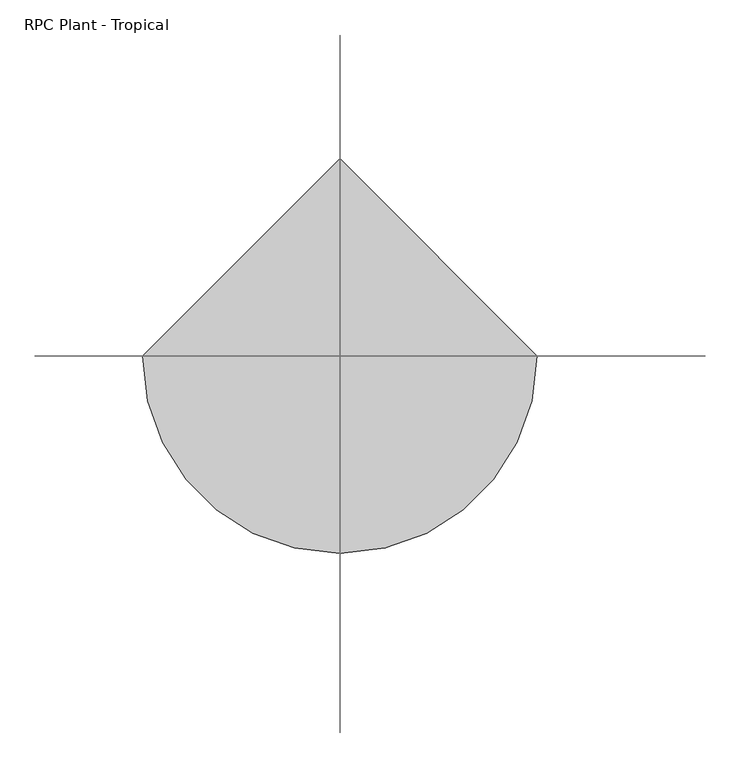
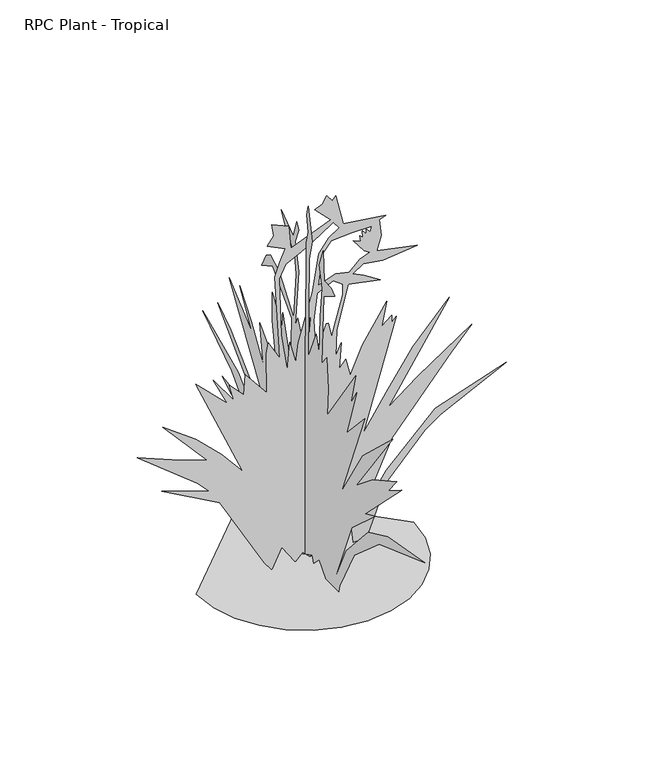
"""IFC4 building model written with IfcOpenShell, lengths in millimetres: geographic element geometry, RPC Plant - Tropical."""

from ifc_helpers import new_model, si_unit, origin, place, context, project, spatial, triangles, source, transform, mapped, element, save


def rpc_plant_tropical_5a024449(model_context):
    return source(origin(), model_context, "Body", "Tessellation", [
        triangles([(-352.4506888, 0.0, 0.0363366), (-343.133961, -80.7585154, 0.0363366), (-316.5967, -154.9221753, 0.0363366), (-274.9660652, -220.3661821, 0.0363366), (-220.3661821, -274.9660652, 0.0363366), (-154.9221753, -316.5967, 0.0363366), (-80.7585154, -343.133961, 0.0363366), (1.54e-05, -352.4506888, 0.0363366), (80.7585154, -343.133961, 0.0363366), (154.9221753, -316.5967, 0.0363366), (220.3661821, -274.9660652, 0.0363366), (274.9660652, -220.3661821, 0.0363366), (316.5967, -154.9221753, 0.0363366), (343.133961, -80.7585154, 0.0363366), (352.4506888, 3.08e-05, 0.0363366), (-4.62e-05, 352.4506888, 0.0363366), (-7e-06, -188.4942358, 0.0), (-3.7e-06, -119.2212567, 0.072664), (-4.19e-05, -79.9125278, 44.364693), (-4.14e-05, -48.5103157, 13.1292711), (-4.04e-05, -40.4507195, 34.8461175), (2.9e-06, 29.5134692, 0.0471628), (-3.66e-05, 46.7858207, 29.9671479), (-3.6e-05, 67.2433383, 18.6432763), (-3.21e-05, 95.7370796, 107.7136924), (7e-06, 122.150729, 0.0282337), (-3.15e-05, 145.3538185, 54.4566279), (-3.22e-05, 150.4477027, 21.3286672), (-2.45e-05, 219.2584009, 179.4152478), (-2e-05, 268.4033662, 254.4167563), (-1.15e-05, 419.8623445, 314.6778128), (-8.6e-06, 464.3123566, 343.8315928), (-1.17e-05, 402.021355, 334.0278671), (-1.57e-05, 328.9766493, 309.2787601), (-9.5e-06, 412.0797526, 393.381984), (1e-06, 573.7356557, 502.2058285), (-1.06e-05, 373.9628205, 412.4692274), (-2.11e-05, 232.7566504, 272.4267398), (-1.31e-05, 320.2214424, 409.8716752), (-4e-07, 490.2271628, 579.950211), (-5.1e-06, 416.7906206, 532.3505728), (-1.51e-05, 280.1801728, 400.4499393), (-2.2e-05, 197.5793099, 294.4509224), (-1.56e-05, 249.5602758, 431.0688189), (5e-07, 426.8795033, 703.7701967), (-8.6e-06, 297.3021655, 594.3503131), (-2e-06, 366.4105199, 712.4096403), (-7.3e-06, 302.3066384, 630.5538082), (-1.36e-05, 233.9534886, 522.3632827), (-8.7e-06, 254.1095984, 654.8193329), (-1.6e-05, 159.0860926, 554.0354047), (-1.04e-05, 183.2709718, 706.1374941), (-7.4e-06, 185.0015529, 801.6720697), (-1.26e-05, 126.6018291, 714.9293266), (-1.12e-05, 124.5318973, 767.1178562), (-1.76e-05, 79.4309438, 617.9316862), (-1.3e-05, 74.9422506, 778.5851068), (-4.9e-06, 181.3398942, 892.1909632), (-3.1e-06, 242.5915333, 859.2623772), (-2.8e-06, 218.5658196, 907.5833376), (-3.4e-06, 196.0532766, 922.0681366), (-6.5e-06, 144.2406234, 895.875622), (-1.33e-05, 64.0625777, 787.2753468), (-9.2e-06, 49.1612298, 945.4327715), (-7e-06, 58.4837167, 1004.946726), (-2.6e-06, 111.6686472, 1072.5920883), (-4e-07, 133.1706141, 1115.5383768), (-4.9e-06, 65.5147783, 1066.5197845), (-3.9e-06, 46.7858207, 1127.0564964), (-5.1e-06, 35.2674194, 1104.0203299), (-5.7e-06, 55.4238608, 1055.069466), (-9.3e-06, 35.7994659, 961.6447906), (-1.43e-05, 55.4238608, 767.1178562), (-1.4e-05, 41.026452, 798.7933937), (-1.71e-05, 12.2314311, 735.4457342), (-1.69e-05, -5.6583455, 769.5562975), (-7.6e-06, -8.3749288, 1087.6424051), (-6.7e-06, -18.0932474, 1129.9351725), (-4.7e-06, -9.2615923, 1183.6781857), (-4.1e-06, -19.4430719, 1219.2010174), (-8.3e-06, -40.4002548, 1110.9765913), (-9.6e-06, -22.855107, 1040.9876947), (-1.95e-05, -19.4430719, 703.7701967), (-1.83e-05, -62.6354346, 807.4327646), (-2.09e-05, -79.9125278, 746.9637812), (-1.71e-05, -85.0409575, 882.7455368), (-1.46e-05, -98.1639664, 984.6876429), (-1.17e-05, -79.9125278, 1055.069466), (-1.13e-05, -91.4305929, 1086.7449308), (-1.09e-05, -102.9486489, 1118.4170528), (-1.41e-05, -108.7076815, 1017.6365765), (-1.59e-05, -147.9066878, 1015.7603828), (-1.73e-05, -168.637163, 1002.06805), (-1.64e-05, -133.7778445, 980.3865973), (-1.57e-05, -106.2777517, 962.7454502), (-2.22e-05, -94.3099411, 726.8063633), (-2.24e-05, -123.1863762, 763.1148302), (-2.58e-05, -131.7434665, 660.5766123), (-2.83e-05, -125.984443, 568.4321277), (-2.85e-05, -284.3569528, 798.7933937), (-3.06e-05, -258.4414743, 689.3734737), (-3.04e-05, -290.1159762, 744.0817623), (-3.3e-05, -235.4056892, 574.1928589), (-3.43e-05, -336.1882367, 683.6127789), (-3.82e-05, -203.7311873, 352.4710001), (-3.78e-05, -325.8775289, 550.7232522), (-4.05e-05, -492.4352766, 708.0950054), (-3.98e-05, -287.2366462, 424.4580305), (-4.17e-05, -380.6345427, 501.4810544), (-4.55e-05, -516.7854255, 575.8116918), (-4.52e-05, -468.6439236, 516.6025515), (-4.71e-05, -542.6155712, 562.8170271), (-4.4e-05, -338.802394, 359.1257901), (-4.58e-05, -393.7782171, 384.1465376), (-4.35e-05, -263.4686565, 265.0881616), (-4.64e-05, -157.658945, 9.8106396), (-4.49e-05, -230.9356314, 167.2679333), (-4.64e-05, -355.769636, 306.2348325), (-4.97e-05, -463.9838519, 356.4029185), (-5.8e-05, -673.0903833, 392.7859085), (-4.92e-05, -416.1708547, 301.7891554), (-4.67e-05, -276.4290936, 178.0792102), (-4.76e-05, -195.0924704, 24.2081495), (156.4407599, 3.08e-05, 0.0540164), (147.1186091, 2.78e-05, 99.2121401), (104.1123133, 3.39e-05, 28.0194403), (74.1534952, 3.32e-05, 61.6417861), (16.7830803, 3.86e-05, 0.0163075), (-6.8943443, 3.9e-05, 24.1987001), (-32.13939, 4.12e-05, 0.0049902), (-75.5809789, 3.96e-05, 64.5211298), (-108.2819807, 4.37e-05, 0.0242217), (-131.9818967, 4.4e-05, 32.1918168), (-277.0556361, 3.5e-05, 288.8520817), (-464.3123566, 3.7e-05, 392.7859085), (-311.6995789, 3.34e-05, 340.9529531), (-348.8032371, 3.27e-05, 380.3771456), (-544.9387942, 3.2e-05, 536.7600057), (-432.90439, 2.98e-05, 490.7182302), (-317.4586023, 2.73e-05, 447.4941607), (-461.4337169, 2.38e-05, 611.6257484), (-354.9737543, 2.38e-05, 533.6239326), (-271.765988, 2.5e-05, 452.9534932), (-202.2786415, 2.69e-05, 369.7497783), (-354.8924729, 1.27e-05, 721.0455957), (-252.5181985, 1.41e-05, 621.3522623), (-297.3021655, 1.05e-05, 715.2882437), (-231.6454718, 1.31e-05, 622.9033304), (-245.4708816, 1.03e-05, 680.7341028), (-199.3989663, 1.12e-05, 631.7831663), (-193.6399246, 7e-06, 698.0128447), (-124.5318973, 9.1e-06, 611.6257484), (-125.4645892, 1.2e-06, 745.9139179), (-118.7732008, -1.3e-06, 781.5179947), (-81.3393302, 1.1e-06, 715.2882437), (-85.8974459, -2.5e-06, 778.2870872), (-97.8195379, -1.51e-05, 999.0640909), (-82.2889543, -1.85e-05, 1044.4149565), (-63.8773237, -2.17e-05, 1084.6486198), (-121.652549, -2.09e-05, 1112.6597734), (-102.0606671, -2.35e-05, 1141.85959), (-107.2551448, -2.56e-05, 1181.7681278), (-53.1866246, -2.66e-05, 1158.7286184), (-46.7858207, -2.23e-05, 1080.984236), (82.791876, -3.1e-05, 1132.8171913), (30.9610326, -3.18e-05, 1184.6468039), (56.5553461, -3.36e-05, 1195.3351049), (71.2741515, -3.57e-05, 1219.2010174), (88.2593112, -3.5e-05, 1195.8464836), (99.6798441, -3.63e-05, 1209.0409544), (124.9047669, -3.11e-05, 1104.1998247), (261.5829613, -3.6e-05, 1085.2209686), (241.1643857, -3.47e-05, 1078.1055599), (247.6434234, -3.16e-05, 1022.4964542), (232.526014, -2.81e-05, 974.442992), (364.9847348, -3.22e-05, 945.6495461), (252.5110768, -2.66e-05, 934.6123564), (189.4235214, -2.44e-05, 944.2101717), (154.7792516, -2.16e-05, 922.6133795), (190.4700055, -2.22e-05, 905.4700945), (244.0440791, -2.24e-05, 870.7804241), (140.4238415, -1.92e-05, 892.113061), (102.7322468, -8.9e-06, 747.339703), (100.0689646, -3.6e-06, 660.5766123), (117.2288819, -6.7e-06, 699.1914064), (111.5866936, -1.2e-06, 611.6257484), (131.7434665, -3.6e-06, 637.5405184), (146.1408799, -7e-07, 577.0715349), (185.2586048, -7.7e-06, 666.3610703), (265.3438509, -1.85e-05, 789.3445518), (249.8031026, -1.31e-05, 709.5309643), (281.4776045, -1.6e-05, 735.4457342), (281.4776045, -1.46e-05, 712.4096403), (295.8750179, -1.61e-05, 726.8063633), (189.3334469, 1.02e-05, 363.9890471), (263.1983969, 1e-07, 478.5499323), (349.8700324, -1.11e-05, 603.7618752), (468.6439236, -2.4e-05, 732.5637154), (269.9592124, 3e-06, 424.4580305), (365.1879564, -5.5e-06, 496.9700289), (540.6343695, -2.01e-05, 614.5043518), (474.2149861, -1.28e-05, 541.0475347), (282.0360734, 9.1e-06, 313.8541712), (175.5771282, 2.77e-05, 79.3862427), (263.306439, 1.6e-05, 211.1110784), (422.7545371, -2e-07, 366.6882282), (652.9328928, -1.49e-05, 444.6154847), (440.209431, 6e-07, 340.3230134), (389.1045925, 5e-06, 303.7012662), (265.6320601, 1.84e-05, 169.4411655), (197.9718186, 2.84e-05, 0.0676572), (152.5051171, -2.99e-05, 1063.2651867), (84.8953359, -2.67e-05, 1059.6481836), (56.4266521, -2.33e-05, 1023.4176189), (42.4789932, -1.67e-05, 922.6133795), (99.5955106, -2.04e-05, 941.7650448), (143.2615316, -2.16e-05, 931.2494076), (177.0767459, -2.5e-05, 963.6090603), (209.4902289, -2.73e-05, 977.3216681), (191.9066365, -2.72e-05, 988.3689589), (156.7607985, -2.84e-05, 1035.0541906), (181.2907874, -2.89e-05, 1024.4065121), (178.2695329, -2.99e-05, 1044.3201221), (187.5906572, -2.98e-05, 1036.1311598), (186.4540987, -3.11e-05, 1057.9480694), (197.9718186, -3.07e-05, 1043.5513464), (198.4063306, -3.17e-05, 1060.2171896), (211.3004019, -3.15e-05, 1047.3139801), (216.3485676, -3.27e-05, 1063.5597908), (48.6623731, -2.71e-05, 1092.001078), (-14.0239612, -2.21e-05, 1054.3684187), (-62.1379314, -1.86e-05, 1031.511747), (-83.7838303, -1.52e-05, 989.2190523), (-76.8587716, -3.8e-06, 793.0800797), (-58.3035451, 3e-06, 666.3373798), (-49.6651689, -2.9e-06, 758.4818281), (-29.5084913, 7e-07, 683.6127789), (-21.1900174, -3.4e-06, 746.4862667), (24.1221968, -1.47e-05, 902.7268753), (44.8185034, -2.32e-05, 1029.605032), (76.8929719, -2.72e-05, 1073.8553106), (111.5866936, -3e-05, 1095.3809589), (91.4305929, -3.07e-05, 1121.2991444), (40.2783372, -1.5e-05, 895.5437382), (29.068629, -9.2e-06, 806.7283745), (34.2422754, -3.3e-06, 704.1156698), (41.1405802, -3.7e-06, 704.9792799), (68.7334726, -9.5e-06, 781.72118), (74.7695323, -9.7e-06, 780.8609854), (86.8413109, -7.2e-06, 730.846669), (92.8773796, -9.1e-06, 757.5775955), (122.1947579, -1.65e-05, 861.0504948), (122.1947579, -1.87e-05, 897.2675428), (91.1525484, -1.87e-05, 920.5475172), (9.23626, -7.6e-06, 793.7946436), (14.4099058, -6.1e-06, 764.4762297), (17.8590253, -8.2e-06, 797.2423256), (20.4458655, -1.06e-05, 836.0467157)], [[15, 16, 1], [14, 15, 1], [14, 1, 2], [13, 14, 2], [13, 2, 3], [13, 3, 4], [12, 13, 4], [11, 12, 4], [11, 4, 5], [11, 5, 6], [11, 6, 7], [11, 7, 8], [11, 8, 9], [11, 9, 10], [46, 47, 48], [119, 120, 121], [35, 36, 37], [106, 107, 108], [39, 40, 41], [39, 41, 42], [101, 102, 103], [111, 112, 113], [105, 106, 108], [44, 45, 46], [113, 114, 115], [54, 55, 56], [103, 104, 105], [99, 100, 101], [109, 110, 111], [89, 90, 91], [118, 119, 121], [31, 32, 33], [46, 48, 49], [44, 46, 49], [79, 80, 81], [78, 79, 81], [66, 67, 68], [27, 28, 29], [52, 53, 54], [88, 89, 91], [87, 88, 91], [49, 50, 51], [58, 59, 60], [99, 101, 103], [25, 26, 27], [83, 84, 85], [109, 111, 113], [108, 109, 113], [96, 97, 98], [68, 69, 70], [68, 70, 71], [38, 39, 42], [38, 42, 43], [65, 66, 68], [65, 68, 71], [65, 71, 72], [64, 65, 72], [64, 72, 73], [63, 64, 73], [118, 121, 122], [117, 118, 122], [117, 122, 123], [116, 117, 123], [73, 74, 75], [116, 123, 17], [116, 17, 18], [58, 60, 61], [58, 61, 62], [57, 58, 62], [57, 62, 63], [77, 78, 81], [77, 81, 82], [76, 77, 82], [76, 82, 83], [75, 76, 83], [92, 93, 94], [19, 20, 21], [30, 31, 33], [30, 33, 34], [91, 92, 94], [87, 91, 94], [87, 94, 95], [86, 87, 95], [86, 95, 96], [85, 86, 96], [34, 35, 37], [34, 37, 38], [30, 34, 38], [25, 27, 29], [57, 63, 73], [56, 57, 73], [56, 73, 75], [56, 75, 83], [23, 24, 25], [99, 103, 105], [29, 30, 38], [105, 108, 113], [105, 113, 115], [51, 52, 54], [51, 54, 56], [83, 85, 96], [21, 22, 23], [83, 96, 98], [83, 98, 99], [56, 83, 99], [29, 38, 43], [25, 29, 43], [115, 116, 18], [115, 18, 19], [105, 115, 19], [21, 23, 25], [44, 49, 51], [43, 44, 51], [56, 99, 105], [51, 56, 105], [43, 51, 105], [43, 105, 19], [25, 43, 19], [21, 25, 19], [248, 124, 125], [241, 229, 212], [206, 207, 208], [197, 198, 199], [146, 147, 148], [134, 135, 136], [196, 197, 199], [241, 212, 213], [255, 237, 238], [140, 141, 142], [200, 201, 202], [137, 138, 139], [255, 238, 239], [258, 255, 239], [175, 176, 177], [184, 185, 186], [235, 236, 237], [180, 181, 182], [189, 190, 191], [144, 145, 146], [140, 142, 143], [247, 248, 125], [171, 172, 173], [200, 202, 203], [199, 200, 203], [193, 194, 195], [237, 255, 256], [220, 221, 222], [148, 149, 150], [137, 139, 140], [224, 225, 226], [229, 241, 242], [195, 196, 199], [222, 223, 224], [153, 154, 155], [179, 180, 182], [150, 151, 152], [226, 227, 228], [191, 192, 193], [186, 187, 188], [169, 170, 171], [175, 177, 178], [152, 153, 155], [195, 199, 203], [161, 162, 163], [240, 241, 213], [240, 213, 214], [165, 166, 167], [167, 168, 169], [165, 167, 169], [165, 169, 171], [191, 193, 195], [189, 191, 195], [188, 189, 195], [239, 240, 214], [239, 214, 215], [125, 126, 127], [124, 248, 249], [124, 249, 250], [161, 163, 164], [160, 161, 164], [159, 160, 164], [131, 132, 133], [144, 146, 148], [129, 130, 131], [131, 133, 134], [206, 208, 209], [205, 206, 209], [205, 209, 210], [204, 205, 210], [204, 210, 211], [204, 211, 124], [204, 124, 250], [246, 247, 125], [195, 203, 204], [144, 148, 150], [144, 150, 152], [158, 159, 164], [127, 128, 129], [246, 125, 127], [246, 127, 129], [246, 129, 131], [136, 137, 140], [136, 140, 143], [136, 143, 144], [134, 136, 144], [131, 134, 144], [220, 222, 224], [220, 224, 226], [220, 226, 228], [219, 220, 228], [131, 144, 152], [258, 239, 215], [174, 175, 178], [186, 188, 195], [215, 216, 217], [131, 152, 155], [157, 158, 164], [217, 218, 219], [186, 195, 204], [219, 228, 229], [245, 246, 131], [245, 131, 215], [244, 245, 215], [254, 244, 215], [254, 215, 217], [253, 254, 217], [252, 253, 217], [257, 258, 215], [184, 186, 204], [184, 204, 250], [183, 184, 250], [183, 250, 251], [182, 183, 251], [182, 251, 252], [182, 252, 217], [179, 182, 217], [179, 217, 219], [178, 179, 219], [174, 178, 219], [174, 219, 229], [173, 174, 229], [171, 173, 229], [171, 229, 242], [165, 171, 242], [165, 242, 243], [165, 243, 230], [164, 165, 230], [164, 230, 231], [164, 231, 232], [157, 164, 232], [157, 232, 233], [156, 157, 233], [156, 233, 234], [156, 234, 235], [155, 156, 235], [131, 155, 235], [131, 235, 237], [131, 237, 256], [215, 131, 256], [257, 215, 256]], closed=False),
    ])


if __name__ == "__main__":
    model = new_model("IFC4")
    model_context = context("Model", 3, world=origin())
    ifc_project = project(units=[si_unit("LENGTHUNIT", "METRE", prefix="MILLI")], contexts=[model_context])
    site = spatial("IfcSite", under=ifc_project)
    building = spatial("IfcBuilding", under=site)
    placement = place(None, origin())
    rpc_plant_tropical_shape = rpc_plant_tropical_5a024449(model_context)
    element("IfcGeographicElement", 1, ObjectType="RPC Plant - Tropical", at=placement, inside=building, context=model_context, shape_type="MappedRepresentation", body=[
        mapped(rpc_plant_tropical_shape, transform((0.0, 0.0, 0.0), x_axis=(1.0, 0.0, 0.0), y_axis=(0.0, 1.0, 0.0), z_axis=(0.0, 0.0, 1.0))),
    ])
    save(model, "model.ifc")

# Revit data of these elements
# Type "RPC Plant - Tropical"
#   built-in parameter 1005198 = "{2, 15},{39, RPC-16-FWM5-GM7X-C67P-4000-ST1L-LVER-AU},{1, 0},{1, 0},{2, 35},{1, 8},{5, Color},{1, 0},{1, 0},{3, 0.8},{3, 0.8},{3, 0.8},{1, 8},{7, BBoxMin},{1, 0},{1, 0},{1, 0},{1, 0},{1, 0},{1, 8},{7, BBoxMax},{1, 0},{1, 0},{1, 0},{1, 0},{1, 0},{2, 11},{9, RPCTypeId},{1, 0},{1, 0},{39, RPC-16-FWM5-GM7X-C67P-4000-ST1L-LVER-AU},{1, 6},{14, RPCPlantHeight},{1, 0},{1, 0},{1, 3},{2, 11},{7, keyword},{1, 0},{1, 0},{99, :Geometry:RPC:Crane Lily:strelitzia:reinae:crane lily:plants:shrub:flower:tropical:bird-of-paradise},{2, 11},{8, category},{1, 0},{1, 0},{17, :Shrubs [General]},{2, 11},{12, LocalizedUID},{1, 0},{1, 0},{10, Crane Lily},{2, 14},{6, Height},{1, 0},{1, 0},{1, 3},{1, 2},{16, Cast Reflections},{1, 0},{1, 0},{1, 0},{1, 2},{12, Cast Shadows},{1, 0},{1, 0},{1, 1},{1, 2},{9, Lock View},{1, 0},{1, 0},{1, 0},{1, 4},{5, ViewC},{1, 0},{1, 0},{1, 0},{2, 11},{20, AdvancedUIDefinition},{1, 0},{1, 0},{0, },{2, 11},{10, AssetLibID},{1, 0},{1, 0},{36, 4D3F6E72-3F99-4203-98E9-AF80B3C7A7A4},{2, 11},{10, BaseSchema},{1, 0},{1, 0},{9, RPCSchema},{2, 11},{12, ExchangeGUID},{1, 0},{1, 0},{0, },{1, 2},{6, Hidden},{1, 0},{1, 0},{1, 0},{1, 4},{11, RPCCategory},{1, 0},{1, 0},{1, 0},{2, 11},{8, RPCImage},{1, 0},{1, 0},{0, },{1, 4},{13, SchemaVersion},{1, 0},{1, 0},{1, 4},{2, 11},{12, UIDefinition},{1, 0},{1, 0},{0, },{2, 11},{6, UIName},{1, 0},{1, 0},{39, RPC-16-FWM5-GM7X-C67P-4000-ST1L-LVER-AU},{2, 11},{11, VersionGUID},{1, 0},{1, 0},{9, RPCSchema},{2, 11},{9, assettype},{1, 0},{1, 0},{11, RPCGeometry},{2, 11},{11, description},{1, 0},{1, 0},{0, },{2, 11},{9, localname},{1, 0},{1, 0},{3, RPC},{2, 11},{9, localtype},{1, 0},{1, 0},{3, RPC},{1, 4},{8, revision},{1, 0},{1, 0},{1, 1},{2, 11},{9, thumbnail},{1, 0},{1, 0},{0, },{1, 4},{7, version},{1, 0},{1, 0},{1, 1},{1, 2},{20, RPC_Cast Reflections},{1, 0},{1, 0},{1, 1},{1, 2},{16, RPC_Cast Shadows},{1, 0},{1, 0},{1, 1},{1, 2},{13, RPC_Lock View},{1, 0},{1, 0},{1, 0},{1, 4},{9, RPC_ViewC},{1, 0},{1, 0},{1, 0},{21, assetlibrary_base.fbx},{1, 5},"
#   built-in parameter 1005195 = "RPC-16-FWM5-GM7X-C67P-4000-ST1L-LVER-AU"
#   Assembly Code = "G2050500"
#   Height = 4' - 0"
#   Default Elevation = 0
